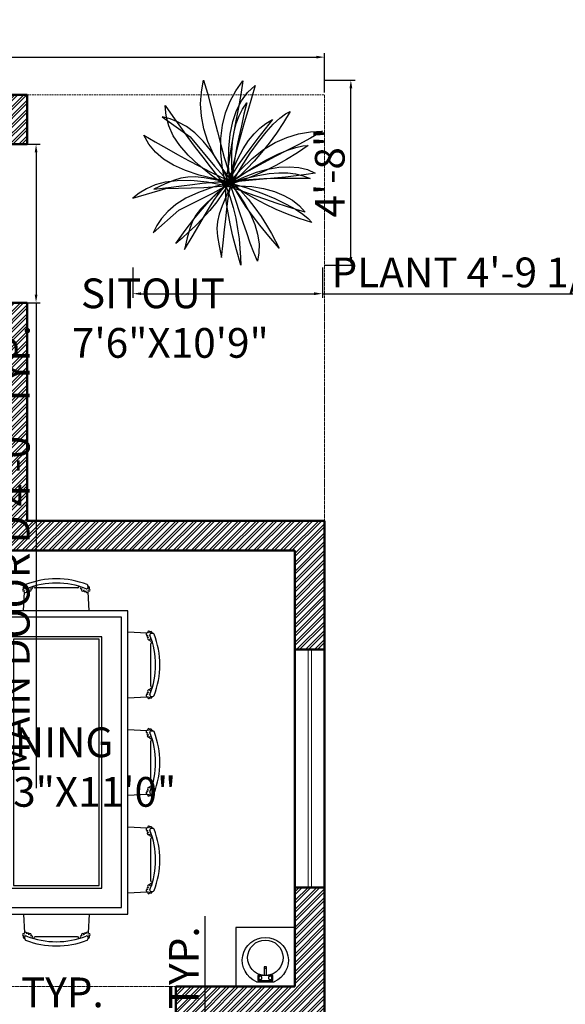
# Model space of a CAD drawing. Units: inches. Extents: x 3590 to 5167, y 65 to 1917.
# Tile 22 of 100: x 4213 to 4378, y 1531 to 1829. Entities that reach past the tile are written whole.
import ezdxf

# ---------------------------------------------------------------- set-up
doc = ezdxf.new("R2010")
doc.units = ezdxf.units.IN
doc.linetypes.add('DASHED', pattern=[0.75, 0.5, -0.25])
for name, color, linetype, lineweight in [('A-ANNO-DIMS', 2, 'Continuous', 18), ('A-AREA-IDEN', 7, 'Continuous', 18), ('A-FLOR-FIXT', 8, 'Continuous', 18), ('A-FURN', 21, 'Continuous', 18), ('A-GLAZ', 4, 'Continuous', 18), ('A-WALL', 7, 'Continuous', 50), ('A-WALL-PATT', 251, 'Continuous', 13), ('L-PLNT', 94, 'Continuous', 18), ('S-BEAM-OVHD', 7, 'DASHED', 18)]:
    doc.layers.add(name, color=color, linetype=linetype, lineweight=lineweight)
for name, color, linetype in [('DIENHOA', 3, 'Continuous'), ('FUR', 42, 'Continuous'), ('HA', 9, 'Continuous'), ('SANTEH', 7, 'Continuous'), ('wood', 26, 'Continuous')]:
    doc.layers.add(name, color=color, linetype=linetype)
doc.styles.get("Standard").update_dxf_attribs({"font": 'arial.ttf'})
doc.dimstyles.new('ISO-25', dxfattribs={"dimtxt": 9, "dimasz": 2.5, "dimexe": 1.25, "dimexo": 0.625, "dimtad": 1, "dimdec": 1, "dimlunit": 3, "dimtxsty": 'Standard', "dimcen": 2.5, "dimadec": 0, "dimazin": 0, "dimtfac": 1, "dimtdec": 1, "dimtmove": 0, "dimatfit": 3, "dimfxl": 1, "dimarcsym": 0})

# ---------------------------------------------------------------- blocks, each defined once
blk = doc.blocks.new('*D5')
at = {"layer": 'A-ANNO-DIMS', "color": 0, "lineweight": -2, "transparency": 16777216}
for p, q in [((3645.51, 1806.62), (3645.51, 1818.61)), ((4305.51, 1806.62), (4305.51, 1818.61)), ((3648.01, 1817.36), (4303.01, 1817.36))]:
    blk.add_line(p, q, dxfattribs=at)
at = {"layer": 'A-ANNO-DIMS', "color": 0, "transparency": 16777216}
for points in [[(3648.01, 1817.78), (3648.01, 1816.95), (3645.51, 1817.36)], [(4303.01, 1817.78), (4303.01, 1816.95), (4305.51, 1817.36)]]:
    blk.add_solid(points, dxfattribs=at)
at = {"layer": 'Defpoints', "color": 0, "transparency": 16777216}
for p in [(4305.51, 1817.36), (3645.51, 1806), (4305.51, 1806)]:
    blk.add_point(p, dxfattribs=at)
at = {"layer": 'A-ANNO-DIMS', "color": 0, "transparency": 16777216, "insert": (3975.51, 1822.57), "char_height": 9, "attachment_point": 5}
blk.add_mtext("55'", dxfattribs=at)
blk = doc.blocks.new('Cay03_mb')
at = {"layer": 'DIENHOA'}
for p, q in [((79.5, 503.7), (118.6, 555.3)), ((118.6, 555.3), (166.2, 599.1)), ((166.2, 599.1), (142.2, 519.4)), ((48.6, 443.6), (79.5, 503.7)), ((142.2, 519.4), (119, 441.7)), ((25.5, 374.3), (48.6, 443.6)), ((119, 441.7), (96.7, 365.6)), ((-365.2, 390.3), (-414.4, 402.8)), ((-414.4, 402.8), (-240.2, 277.8)), ((-314.9, 371.3), (-365.2, 390.3)), ((-263.5, 343.5), (-314.9, 371.3)), ((9.9, 295.3), (25.5, 374.3)), ((-211.2, 304.6), (-263.5, 343.5)), ((96.7, 365.6), (75.6, 290.6)), ((436.8, 297.2), (511, 309.6)), ((511, 309.6), (585.9, 313.5)), ((585.9, 313.5), (511.8, 271.4)), ((-240.2, 277.8), (-88.4, 94.9)), ((-158, 252.3), (-211.2, 304.6)), ((-104.2, 184.4), (-158, 252.3)), ((1.6, 205.7), (9.9, 295.3)), ((75.6, 290.6), (55.7, 216.3)), ((290.6, 243.2), (363.4, 275.4)), ((363.4, 275.4), (436.8, 297.2)), ((511.8, 271.4), (437.6, 231.5)), ((0.2, 104.9), (1.6, 205.7)), ((55.7, 216.3), (37.3, 142.1)), ((147, 144.1), (218.5, 199.8)), ((218.5, 199.8), (290.6, 243.2)), ((363.7, 192.9), (290.2, 154.9)), ((437.6, 231.5), (363.7, 192.9)), ((-49.6, 98.5), (-104.2, 184.4)), ((37.3, 142.1), (20.5, 67.6)), ((75.9, 75.2), (147, 144.1)), ((290.2, 154.9), (217.4, 116.6)), ((-88.4, 94.9), (5.4, -7.8)), ((5.4, -7.8), (-49.6, 98.5)), ((5.4, -7.8), (0.2, 104.9)), ((5.4, -7.8), (75.9, 75.2)), ((20.5, 67.6), (5.4, -7.8)), ((145.5, 77.3), (74.7, 36.1)), ((217.4, 116.6), (145.5, 77.3)), ((-345, 5.4), (-399.6, -17.1)), ((-298.6, 20.1), (-345, 5.4)), ((-254.7, 27.4), (-298.6, 20.1)), ((-208, 27.8), (-254.7, 27.4)), ((-152.7, 21.7), (-208, 27.8)), ((-83.4, 9.7), (-152.7, 21.7)), ((5.4, -7.8), (-83.4, 9.7)), ((74.7, 36.1), (5.4, -7.8)), ((5.4, -7.8), (100.3, 18.4)), ((46.3, 0.9), (5.4, -7.8)), ((96.7, 7.5), (46.3, 0.9)), ((155, 12.2), (96.7, 7.5)), ((100.3, 18.4), (182.2, 37.2)), ((219.6, 15.4), (155, 12.2)), ((182.2, 37.2), (253, 48.9)), ((289, 17.4), (219.6, 15.4)), ((253, 48.9), (314.6, 54.1)), ((361.6, 18.5), (289, 17.4)), ((314.6, 54.1), (369.2, 53.3)), ((435.8, 18.9), (361.6, 18.5)), ((369.2, 53.3), (418.6, 46.8)), ((418.6, 46.8), (464.9, 35.2)), ((510, 19), (435.8, 18.9)), ((464.9, 35.2), (510, 19)), ((-399.6, -17.1), (-468, -47.9)), ((-468, -47.9), (-375.6, -37.8)), ((-375.6, -37.8), (-295.3, -27.9)), ((-295.3, -27.9), (-225.8, -18.9)), ((-225.8, -18.9), (-165.8, -11.3)), ((-165.8, -11.3), (-114, -5.7)), ((-114, -5.7), (-69, -2.9)), ((-79.8, -79.6), (-45.1, -46.3)), ((-69, -2.9), (-29.6, -3.4)), ((-45.1, -46.3), (-16.5, -22.4)), ((5.4, -7.8), (-33.2, -69.5)), ((-29.6, -3.4), (5.4, -7.8)), ((-16.5, -22.4), (5.4, -7.8)), ((5.4, -7.8), (56.8, -73.3)), ((25.9, -64.4), (5.4, -7.8)), ((5.4, -7.8), (112.8, -40.3)), ((53.5, -41.6), (5.4, -7.8)), ((107, -75.7), (53.5, -41.6)), ((112.8, -40.3), (207.5, -73.8)), ((-165.9, -174.1), (-120.2, -122.1)), ((-120.2, -122.1), (-79.8, -79.6)), ((-33.2, -69.5), (-74.6, -127.3)), ((47, -125.9), (25.9, -64.4)), ((56.8, -73.3), (100.4, -139.1)), ((165.5, -109.6), (107, -75.7)), ((228.7, -142.8), (165.5, -109.6)), ((207.5, -73.8), (289.5, -107.6)), ((289.5, -107.6), (359.3, -141.1)), ((-216.3, -235.6), (-165.9, -174.1)), ((-117.8, -181.1), (-162.1, -230.9)), ((-74.6, -127.3), (-117.8, -181.1)), ((68.7, -190.6), (47, -125.9)), ((100.4, -139.1), (135.9, -204.3)), ((296, -174.7), (228.7, -142.8)), ((367.1, -204.8), (296, -174.7)), ((359.3, -141.1), (416.9, -173.5)), ((416.9, -173.5), (462.6, -204.2)), ((-271, -306.6), (-216.3, -235.6)), ((-162.1, -230.9), (-206.3, -276.5)), ((90.8, -256.6), (68.7, -190.6)), ((135.9, -204.3), (162.8, -268.3)), ((441.6, -232.7), (367.1, -204.8)), ((518.9, -257.7), (441.6, -232.7)), ((462.6, -204.2), (496.5, -232.5)), ((496.5, -232.5), (518.9, -257.7)), ((-329.5, -387.1), (-271, -306.6)), ((-206.3, -276.5), (-249.6, -317.8)), ((113.1, -322.2), (90.8, -256.6)), ((162.8, -268.3), (181, -330.4)), ((-291, -354.7), (-329.5, -387.1)), ((-249.6, -317.8), (-291, -354.7)), ((135.4, -385.6), (113.1, -322.2)), ((181, -330.4), (190, -390)), ((157.6, -445), (135.4, -385.6)), ((190, -390), (189.6, -446.3)), ((179.5, -498.7), (157.6, -445)), ((189.6, -446.3), (179.5, -498.7))]:
    blk.add_line(p, q, dxfattribs=at)
for points in [[(23.7, -5.4), (-41, 82.2), (-91.8, 167.1), (-129.7, 249.5), (-155.6, 329.6), (-170.2, 407.8), (-174.7, 484.2), (-169.8, 559.3), (-156.5, 633.1)], [(-156.5, 633.1), (-132.5, 551.3), (-110.5, 470), (-89.8, 389.2), (-69.6, 309), (-49, 229.4), (-27.1, 150.4), (-3.2, 72.1), (23.7, -5.4)], [(-16.4, -26.7), (-38.3, 80), (-48.9, 178.3), (-48.7, 269), (-38.5, 352.6), (-19.1, 429.7), (9, 501), (44.9, 567.1), (87.9, 628.5)], [(87.9, 628.5), (75.5, 544.2), (61.3, 461.2), (46.1, 379.1), (30.8, 297.8), (16.1, 216.9), (2.9, 136), (-8.3, 54.9), (-16.4, -26.7)], [(-395.6, 473.7), (-347.5, 405.6), (-300.6, 339.5), (-254.3, 275.1), (-208.3, 212.3), (-161.9, 150.9), (-114.8, 90.7), (-66.5, 31.6), (-16.4, -26.7)], [(-16.4, -26.7), (-108.3, 38.6), (-186.9, 101.7), (-252.4, 163.5), (-305.1, 224.4), (-345.4, 285.2), (-373.7, 346.6), (-390.4, 409.2), (-395.6, 473.7)], [(23.7, -5.4), (19.8, 93), (20.3, 177), (25, 248.5), (34, 309.8), (47.3, 362.7), (64.9, 409.3), (86.8, 451.7), (112.9, 491.9)], [(112.9, 491.9), (96, 419.7), (79.5, 347.4), (63.9, 276.5), (50, 208.4), (38.4, 144.8), (29.7, 86.9), (24.6, 36.3), (23.7, -5.4)], [(384.3, 437.5), (342.2, 367.8), (298.1, 301.7), (252.6, 239.4), (206.1, 181.1), (159.4, 127.2), (113, 78), (67.6, 33.6), (23.7, -5.4)], [(23.7, -5.4), (79.9, 91.7), (134.1, 176.2), (185.8, 248.4), (234.3, 308.7), (279, 357.3), (319.3, 394.8), (354.6, 421.4), (384.3, 437.5)], [(273.2, 387.3), (227.6, 328.8), (182.3, 270.1), (138.4, 212.3), (97.2, 156.4), (60, 103.4), (27.8, 54.6), (1.9, 10.8), (-16.4, -26.7)], [(-16.4, -26.7), (21.4, 64.2), (57, 140.3), (91.4, 203.3), (125.2, 255.1), (159.5, 297.5), (195, 332.5), (232.7, 361.8), (273.2, 387.3)], [(-530.5, 289.7), (-458.3, 248.1), (-387.9, 207.8), (-318.9, 168.7), (-250.8, 131.1), (-182.9, 94.8), (-114.9, 59.9), (-46.2, 26.5), (23.7, -5.4)], [(23.7, -5.4), (-87.2, 15.2), (-185, 39.6), (-270.3, 68.2), (-343.7, 101.4), (-405.9, 139.7), (-457.3, 183.5), (-498.7, 233.4), (-530.5, 289.7)], [(496.7, 224), (429.4, 178.4), (361.6, 136.9), (294.1, 99.5), (227.5, 66.1), (162.4, 36.7), (99.7, 11.5), (39.8, -9.7), (-16.4, -26.7)], [(-16.4, -26.7), (75.4, 37.9), (160.1, 91.8), (237.3, 135.7), (306.6, 170), (367.6, 195.4), (419.9, 212.5), (463.1, 221.9), (496.7, 224)], [(23.7, -5.4), (99.3, 29.7), (173.2, 57.1), (244.8, 76.7), (313.3, 88.3), (377.9, 91.8), (437.9, 87), (492.7, 73.8), (541.4, 52)], [(-16.4, -26.7), (-134, -4.7), (-235.3, 5.3), (-322, 4.7), (-395.9, -5), (-458.7, -22.3), (-512.3, -45.7), (-558.2, -73.6), (-598.4, -104.7)], [(541.4, 52), (484.1, 42.9), (421.2, 34.8), (354.4, 27.6), (285.4, 20.9), (216.1, 14.5), (148.2, 8.1), (83.5, 1.6), (23.7, -5.4)], [(-598.4, -104.7), (-392.7, -44.4), (-155, -37.4), (-16.4, -26.7)], [(-471.9, -320.3), (-310.5, -179.3), (-97.7, -73.3), (23.7, -5.4)], [(23.7, -5.4), (-92.3, -34.8), (-188.4, -68.2), (-266.9, -105.1), (-329.9, -144.9), (-379.7, -187), (-418.5, -230.7), (-448.5, -275.3), (-471.9, -320.3)], [(-276.2, -424.4), (-227.3, -345.4), (-185.7, -276.1), (-150, -215.7), (-119.1, -163.8), (-91.5, -119.5), (-66, -82.3), (-41.4, -51.6), (-16.4, -26.7)], [(-16.4, -26.7), (-84.9, -86), (-137, -133.1), (-175.8, -173), (-204.3, -210), (-225.5, -249.1), (-242.5, -294.7), (-258.4, -351.6), (-276.2, -424.4)], [(23.7, -5.4), (-13.6, -87.9), (-41.1, -152.6), (-59.6, -205), (-69.9, -250.7), (-72.8, -295), (-69.2, -343.6), (-59.7, -401.9), (-45.3, -475.5)], [(-45.3, -475.5), (-34.1, -383.2), (-25.4, -302.8), (-18.3, -233.1), (-12, -172.9), (-5.6, -121.2), (2, -76.8), (11.4, -38.5), (23.7, -5.4)], [(76.2, -524.2), (48.8, -428.5), (26.6, -341.7), (9.2, -264.1), (-3.6, -196.1), (-12.3, -138), (-17.1, -90.2), (-18.3, -53), (-16.4, -26.7)], [(-16.4, -26.7), (66.9, -26.6), (145.6, -32.7), (218.8, -44.9), (285.8, -63.1), (345.9, -87.1), (398.4, -116.6), (442.6, -151.6), (477.6, -191.8)], [(477.6, -191.8), (421.8, -176), (361.3, -156.9), (297.6, -135.5), (232.2, -112.6), (166.6, -89.4), (102.3, -66.6), (40.8, -45.4), (-16.4, -26.7)], [(-16.4, -26.7), (8.5, -95.1), (28.5, -163.3), (44.3, -230.6), (56.3, -296.1), (65, -359), (70.9, -418.5), (74.5, -473.9), (76.2, -524.2)], [(316.5, -418.1), (251.4, -342.8), (194.8, -273.3), (146.5, -210.2), (106.3, -153.8), (74.1, -104.7), (49.7, -63.4), (32.9, -30.1), (23.7, -5.4)], [(23.7, -5.4), (74.9, -57.1), (121.8, -110.6), (164.3, -165), (202.7, -219.4), (237, -272.9), (267.3, -324.5), (293.7, -373.2), (316.5, -418.1)]]:
    blk.add_lwpolyline(points, dxfattribs=at)
blk = doc.blocks.new('A$C39F63D19')
at = {"layer": 'FUR'}
for p, q in [((1.415, 2.4468), (1.4061, 2.4547)), ((1.5486, 2.3264), (1.4408, 2.4235)), ((1.3599, 2.3864), (1.1308, 2.1573)), ((1.3599, 2.4017), (1.3588, 2.4028)), ((2.0077, 2.3522), (2.0166, 2.3602)), ((1.8741, 2.2319), (1.9819, 2.329)), ((2.0628, 2.3072), (2.0639, 2.3083)), ((2.0628, 2.2919), (2.2919, 2.0628)), ((1.1155, 2.1573), (1.1144, 2.1585)), ((1.1155, 2.1573), (1.1144, 2.1585)), ((1.0705, 2.1023), (1.0625, 2.1111)), ((1.1908, 1.9686), (1.0937, 2.0765)), ((2.3072, 2.0628), (2.3083, 2.0639)), ((2.3072, 2.0628), (2.3083, 2.0639)), ((2.2319, 1.8741), (2.329, 1.9819)), ((2.3522, 2.0077), (2.3602, 2.0166)), ((0.8846, 1.9165), (0.8758, 1.9244)), ((1.0183, 1.7961), (0.9104, 1.8932)), ((0.8296, 1.8561), (0.6005, 1.627)), ((0.8296, 1.8714), (0.8285, 1.8725)), ((0.5852, 1.627), (0.5841, 1.6281)), ((0.5852, 1.627), (0.5841, 1.6281)), ((0.5401, 1.572), (0.5322, 1.5808)), ((0.6605, 1.4383), (0.5634, 1.5462)), ((2.3264, 1.5486), (2.4235, 1.4408)), ((0.3543, 1.3861), (0.3455, 1.3941)), ((0.488, 1.2658), (0.3801, 1.3629)), ((2.4468, 1.415), (2.4547, 1.4061)), ((0.2993, 1.3258), (0.0701, 1.0967)), ((0.2993, 1.3411), (0.2981, 1.3422)), ((2.3864, 1.3599), (2.1573, 1.1308)), ((2.4017, 1.3599), (2.4028, 1.3588)), ((1.9686, 1.1908), (2.0765, 1.0937)), ((0.0549, 1.0967), (0.0538, 1.0978)), ((0.0549, 1.0967), (0.0538, 1.0978)), ((2.1023, 1.0705), (2.1111, 1.0625)), ((2.1573, 1.1155), (2.1585, 1.1144)), ((2.1573, 1.1155), (2.1585, 1.1144)), ((0.0098, 1.0416), (0.0019, 1.0505)), ((0.1302, 0.908), (0.033, 1.0158)), ((1.7961, 1.0183), (1.8932, 0.9104)), ((1.9165, 0.8846), (1.9244, 0.8758)), ((1.8561, 0.8296), (1.627, 0.6005)), ((1.8714, 0.8296), (1.8725, 0.8285)), ((1.4383, 0.6605), (1.5462, 0.5634)), ((0.2247, 0.5825), (0.1276, 0.4747)), ((1.572, 0.5401), (1.5808, 0.5322)), ((1.627, 0.5852), (1.6281, 0.5841)), ((1.627, 0.5852), (1.6281, 0.5841)), ((1.2658, 0.488), (1.3629, 0.3801)), ((0.1044, 0.4489), (0.0964, 0.44)), ((0.1494, 0.3938), (0.1483, 0.3927)), ((0.1647, 0.3938), (0.3938, 0.1647)), ((1.3861, 0.3543), (1.3941, 0.3455)), ((1.3258, 0.2993), (1.0967, 0.0701)), ((1.3411, 0.2993), (1.3422, 0.2981)), ((0.5825, 0.2247), (0.4747, 0.1276)), ((0.3938, 0.1494), (0.3927, 0.1483)), ((0.3938, 0.1494), (0.3927, 0.1483)), ((0.4489, 0.1044), (0.44, 0.0964)), ((0.908, 0.1302), (1.0158, 0.033)), ((1.0416, 0.0098), (1.0505, 0.0019)), ((1.0967, 0.0549), (1.0978, 0.0538)), ((1.0967, 0.0549), (1.0978, 0.0538))]:
    blk.add_line(p, q, dxfattribs=at)
for points in [[(1.6641, 2.4419), (0.0147, 0.7925), (0.7925, 0.0147), (2.4419, 1.6641)], [(1.6641, 2.3712), (0.0854, 0.7925), (0.7925, 0.0854), (2.3712, 1.6641)], [(1.6641, 2.159), (0.2976, 0.7925), (0.7925, 0.2976), (2.159, 1.6641)]]:
    blk.add_lwpolyline(points, close=True, dxfattribs=at)
for centre, radius, start, end in [((1.6574, 1.8598), 0.6521, 113.77302, 156.22698), ((1.6574, 1.8598), 0.6197, 113.33062, 156.66938), ((1.3989, 2.4467), 0.0108, 48, 113.77302), ((1.4185, 2.4458), 0.0101, 329.62103, 147.42526), ((1.4077, 2.4388), 0.0108, 293.33062, 48), ((1.4308, 2.4208), 0.0103, 213.3009, 71.36297), ((1.4349, 2.4385), 0.00795, 264.76881, 163.65384), ((1.3523, 2.3941), 0.0108, 315, 45), ((1.3814, 2.4068), 0.0085, 151.04971, 5.85435), ((1.3995, 2.4044), 0.0102, 161.25601, 35.99509), ((1.4156, 2.411), 0.00785, 184.4301, 31.81325), ((1.9878, 2.3439), 0.00795, 16.34616, 275.23119), ((2.0042, 2.3512), 0.0101, 32.57474, 210.37897), ((2.015, 2.3442), 0.0108, 132, 246.66938), ((2.0238, 2.3521), 0.0108, 66.22698, 132), ((1.7653, 1.7653), 0.6521, 23.77302, 66.22698), ((1.9919, 2.3262), 0.0103, 108.63703, 326.6991), ((2.0071, 2.3164), 0.00785, 148.18675, 355.5699), ((1.7653, 1.7653), 0.6197, 23.33062, 66.66938), ((2.0232, 2.3098), 0.0102, 144.00491, 18.74399), ((2.0413, 2.3122), 0.0085, 174.14565, 28.95029), ((2.0704, 2.2995), 0.0108, 135, 225), ((1.0705, 2.1184), 0.0108, 156.22698, 222), ((1.1105, 2.1359), 0.0085, 264.14565, 118.95029), ((1.1232, 2.165), 0.0108, 225, 315), ((1.0715, 2.0987), 0.0101, 122.57474, 300.37897), ((1.0785, 2.1095), 0.0108, 222, 336.66938), ((1.0788, 2.0824), 0.00795, 106.34616, 5.23119), ((1.0965, 2.0864), 0.0103, 198.63703, 56.6991), ((1.1063, 2.1017), 0.00785, 238.18675, 85.5699), ((2.2995, 2.0704), 0.0108, 225, 315), ((2.3122, 2.0413), 0.0085, 61.04971, 275.85435), ((2.3098, 2.0232), 0.0102, 71.25601, 305.99509), ((2.3164, 2.0071), 0.00785, 94.4301, 301.81325), ((2.3262, 1.9919), 0.0103, 123.3009, 341.36297), ((2.3442, 2.015), 0.0108, 203.33062, 318), ((2.3439, 1.9878), 0.00795, 174.76881, 73.65384), ((2.3512, 2.0042), 0.0101, 239.62103, 57.42526), ((2.3521, 2.0238), 0.0108, 318, 23.77302), ((1.1271, 1.3295), 0.6521, 113.77302, 156.22698), ((1.1271, 1.3295), 0.6197, 113.33062, 156.66938), ((0.8686, 1.9164), 0.0108, 48, 113.77302), ((0.8882, 1.9155), 0.0101, 329.62103, 147.42526), ((0.8774, 1.9084), 0.0108, 293.33062, 48), ((0.9005, 1.8904), 0.0103, 213.3009, 71.36297), ((0.9045, 1.9081), 0.00795, 264.76881, 163.65384), ((0.8219, 1.8638), 0.0108, 315, 45), ((0.8511, 1.8765), 0.0085, 151.04971, 5.85435), ((0.8692, 1.8741), 0.0102, 161.25601, 35.99509), ((0.8852, 1.8806), 0.00785, 184.4301, 31.81325), ((0.5402, 1.588), 0.0108, 156.22698, 222), ((0.5801, 1.6055), 0.0085, 264.14565, 118.95029), ((0.5825, 1.5874), 0.0102, 234.00491, 108.74399), ((0.5928, 1.6347), 0.0108, 225, 315), ((0.5411, 1.5684), 0.0101, 122.57474, 300.37897), ((0.5482, 1.5792), 0.0108, 222, 336.66938), ((0.5485, 1.5521), 0.00795, 106.34616, 5.23119), ((0.5662, 1.5561), 0.0103, 198.63703, 56.6991), ((0.576, 1.5714), 0.00785, 238.18675, 85.5699), ((2.4208, 1.4308), 0.0103, 18.63703, 236.6991), ((2.4385, 1.4349), 0.00795, 286.34616, 185.23119), ((0.5968, 0.7992), 0.6521, 113.77302, 156.22698), ((0.5968, 0.7992), 0.6197, 113.33062, 156.66938), ((0.3382, 1.3861), 0.0108, 48, 113.77302), ((0.3579, 1.3851), 0.0101, 329.62103, 147.42526), ((0.3471, 1.3781), 0.0108, 293.33062, 48), ((0.3702, 1.3601), 0.0103, 213.3009, 71.36297), ((0.3742, 1.3778), 0.00795, 264.76881, 163.65384), ((1.8598, 1.6574), 0.6197, 293.33062, 336.66938), ((1.8598, 1.6574), 0.6521, 293.77302, 336.22698), ((2.3941, 1.3523), 0.0108, 45, 135), ((2.4044, 1.3995), 0.0102, 54.00491, 288.74399), ((2.4068, 1.3814), 0.0085, 84.14565, 298.95029), ((2.411, 1.4156), 0.00785, 58.18675, 265.5699), ((2.4388, 1.4077), 0.0108, 42, 156.66938), ((2.4458, 1.4185), 0.0101, 302.57474, 120.37897), ((2.4467, 1.3989), 0.0108, 336.22698, 42), ((0.2916, 1.3334), 0.0108, 315, 45), ((0.3207, 1.3461), 0.0085, 151.04971, 5.85435), ((0.3388, 1.3437), 0.0102, 161.25601, 35.99509), ((0.3549, 1.3503), 0.00785, 184.4301, 31.81325), ((0.0099, 1.0577), 0.0108, 156.22698, 222), ((0.0498, 1.0752), 0.0085, 264.14565, 118.95029), ((0.0522, 1.0571), 0.0102, 234.00491, 108.74399), ((0.0625, 1.1043), 0.0108, 225, 315), ((2.0824, 1.0788), 0.00795, 84.76881, 343.65384), ((2.0864, 1.0965), 0.0103, 33.3009, 251.36297), ((2.0987, 1.0715), 0.0101, 149.62103, 327.42526), ((2.1017, 1.1063), 0.00785, 4.4301, 211.81325), ((2.1095, 1.0785), 0.0108, 113.33062, 228), ((2.1178, 1.1129), 0.0102, 341.25601, 215.99509), ((2.1184, 1.0705), 0.0108, 228, 293.77302), ((2.1359, 1.1105), 0.0085, 331.04971, 185.85435), ((2.165, 1.1232), 0.0108, 135, 225), ((0.0108, 1.0381), 0.0101, 122.57474, 300.37897), ((0.0178, 1.0489), 0.0108, 222, 336.66938), ((0.0181, 1.0217), 0.00795, 106.34616, 5.23119), ((0.0358, 1.0258), 0.0103, 198.63703, 56.6991), ((0.0456, 1.041), 0.00785, 238.18675, 85.5699), ((1.8904, 0.9005), 0.0103, 18.63703, 236.6991), ((1.9081, 0.9045), 0.00795, 286.34616, 185.23119), ((1.3295, 1.1271), 0.6197, 293.33062, 336.66938), ((1.3295, 1.1271), 0.6521, 293.77302, 336.22698), ((1.8741, 0.8692), 0.0102, 54.00491, 288.74399), ((1.8765, 0.8511), 0.0085, 84.14565, 298.95029), ((1.8806, 0.8852), 0.00785, 58.18675, 265.5699), ((1.9084, 0.8774), 0.0108, 42, 156.66938), ((1.9155, 0.8882), 0.0101, 302.57474, 120.37897), ((1.9164, 0.8686), 0.0108, 336.22698, 42), ((1.8638, 0.8219), 0.0108, 45, 135), ((1.5521, 0.5485), 0.00795, 84.76881, 343.65384), ((1.5561, 0.5662), 0.0103, 33.3009, 251.36297), ((1.5684, 0.5411), 0.0101, 149.62103, 327.42526), ((1.5714, 0.576), 0.00785, 4.4301, 211.81325), ((1.5792, 0.5482), 0.0108, 113.33062, 228), ((1.5874, 0.5825), 0.0102, 341.25601, 215.99509), ((1.588, 0.5402), 0.0108, 228, 293.77302), ((1.6055, 0.5801), 0.0085, 331.04971, 185.85435), ((1.6347, 0.5928), 0.0108, 135, 225), ((0.1054, 0.4524), 0.0101, 59.62103, 237.42526), ((0.1127, 0.4688), 0.00795, 354.76881, 253.65384), ((0.1304, 0.4647), 0.0103, 303.3009, 161.36297), ((0.1402, 0.4495), 0.00785, 274.4301, 121.81325), ((0.1044, 0.4328), 0.0108, 138, 203.77302), ((0.6913, 0.6913), 0.6521, 203.77302, 246.22698), ((0.1124, 0.4416), 0.0108, 23.33062, 138), ((0.6913, 0.6913), 0.6197, 203.33062, 246.66938), ((0.1444, 0.4153), 0.0085, 241.04971, 95.85435), ((0.1468, 0.4334), 0.0102, 251.25601, 125.99509), ((0.1571, 0.3862), 0.0108, 45, 135), ((1.3601, 0.3702), 0.0103, 18.63703, 236.6991), ((1.3778, 0.3742), 0.00795, 286.34616, 185.23119), ((0.7992, 0.5968), 0.6197, 293.33062, 336.66938), ((0.7992, 0.5968), 0.6521, 293.77302, 336.22698), ((1.3437, 0.3388), 0.0102, 54.00491, 288.74399), ((1.3461, 0.3207), 0.0085, 84.14565, 298.95029), ((1.3503, 0.3549), 0.00785, 58.18675, 265.5699), ((1.3781, 0.3471), 0.0108, 42, 156.66938), ((1.3851, 0.3579), 0.0101, 302.57474, 120.37897), ((1.3861, 0.3382), 0.0108, 336.22698, 42), ((1.3334, 0.2916), 0.0108, 45, 135), ((0.3862, 0.1571), 0.0108, 315, 45), ((0.4153, 0.1444), 0.0085, 354.14565, 208.95029), ((0.4334, 0.1468), 0.0102, 324.00491, 198.74399), ((0.4328, 0.1044), 0.0108, 246.22698, 312), ((0.4495, 0.1402), 0.00785, 328.18675, 175.5699), ((0.4524, 0.1054), 0.0101, 212.57474, 30.37897), ((0.4416, 0.1124), 0.0108, 312, 66.66938), ((0.4647, 0.1304), 0.0103, 288.63703, 146.6991), ((0.4688, 0.1127), 0.00795, 196.34616, 95.23119), ((1.0217, 0.0181), 0.00795, 84.76881, 343.65384), ((1.0258, 0.0358), 0.0103, 33.3009, 251.36297), ((1.0381, 0.0108), 0.0101, 149.62103, 327.42526), ((1.041, 0.0456), 0.00785, 4.4301, 211.81325), ((1.0489, 0.0178), 0.0108, 113.33062, 228), ((1.0571, 0.0522), 0.0102, 341.25601, 215.99509), ((1.0577, 0.0099), 0.0108, 228, 293.77302), ((1.0752, 0.0498), 0.0085, 331.04971, 185.85435), ((1.1043, 0.0625), 0.0108, 135, 225)]:
    blk.add_arc(centre, radius, start, end, dxfattribs=at)
at = {"layer": 'HA'}
blk.add_lwpolyline([(1.6641, 2.1308), (0.3258, 0.7925), (0.7925, 0.3258), (2.1308, 1.6641)], close=True, dxfattribs=at)
at = {"layer": 'wood'}
for points in [[(1.3825, 2.4152, 0.308332), (1.374, 2.4109, -0.00386)], [(1.4096, 2.4059, -0.15729), (1.4077, 2.4104, -0.120016)], [(1.1113, 2.1077, 1.044756), (1.1135, 2.1279, -0.117685), (1.1096, 2.1274, -1.643727), (1.1069, 2.1095, -0.15729)], [(2.3158, 2.015, -0.120016), (2.3113, 2.0131, -0.15729)], [(0.8522, 1.8849, 0.308332), (0.8436, 1.8806, -0.00386)], [(0.8792, 1.8756, -0.15729), (0.8774, 1.88, -0.120016)], [(0.581, 1.5774, 1.044756), (0.5832, 1.5976, -0.117685), (0.5793, 1.5971, -1.643727), (0.5766, 1.5792, -0.15729)], [(2.4104, 1.4077, -0.15729), (2.4059, 1.4096, 1.044756), (2.4037, 1.3893, -0.117685), (2.4077, 1.3899, -1.643727)], [(0.3489, 1.3453, -0.15729), (0.3471, 1.3497, -0.120016)], [(2.1095, 1.1069, -0.120016), (2.1077, 1.1113, -0.15729)], [(2.1347, 1.102, 0.308332), (2.1433, 1.1064, -0.00386)], [(1.88, 0.8774, -0.15729), (1.8756, 0.8792, 1.044756), (1.8734, 0.859, -0.117685), (1.8773, 0.8595, -1.643727)], [(1.5792, 0.5766, -0.120016), (1.5774, 0.581, -0.15729)], [(1.6044, 0.5717, 0.308332), (1.613, 0.576, -0.00386)], [(0.1453, 0.4435, -0.15729), (0.1408, 0.4416, -0.120016)], [(1.3497, 0.3471, -0.15729), (1.3453, 0.3489, 1.044756), (1.3431, 0.3287, -0.117685), (1.347, 0.3292, -1.643727)], [(1.0489, 0.0462, -0.120016), (1.047, 0.0507, -0.15729)], [(1.0741, 0.0414, 0.308332), (1.0826, 0.0457, -0.00386)]]:
    blk.add_lwpolyline(points, format="xyb", close=True, dxfattribs=at)
blk = doc.blocks.new('r11')
at = {"layer": 'SANTEH', "ltscale": 5}
for p, q in [((0, 0), (600, 0)), ((0, -600), (0, 0)), ((600, 0), (600, -600)), ((210, -50), (390, -50)), ((210, -50), (210, -50)), ((224, -63), (376, -63)), ((224, -113), (224, -63)), ((233, -79), (249, -69)), ((233, -98), (233, -79)), ((249, -107), (233, -98)), ((249, -69), (266, -79)), ((266, -98), (249, -107)), ((266, -79), (266, -98)), ((334, -79), (351, -69)), ((334, -98), (334, -79)), ((351, -107), (334, -98)), ((351, -69), (367, -79)), ((367, -98), (351, -107)), ((367, -79), (367, -98)), ((376, -63), (376, -113)), ((376, -113), (224, -113)), ((288, -202), (288, -113)), ((312, -184), (288, -184)), ((312, -113), (312, -202)), ((312, -202), (288, -202)), ((600, -600), (0, -600))]:
    blk.add_line(p, q, dxfattribs=at)
for centre, radius, start, end in [((300, -266), 234, 112.5, 67.5), ((300, -293), 180, 93.8183, 86.1817)]:
    blk.add_arc(centre, radius, start, end, dxfattribs=at)
blk = doc.blocks.new('*D294')
at = {"layer": 'A-ANNO-DIMS', "color": 0, "lineweight": -2, "transparency": 16777216}
for p, q in [((3946.19, 1546.03), (3946.19, 1526.56)), ((4071.76, 1546.03), (4071.76, 1526.56)), ((3948.69, 1527.81), (4069.26, 1527.81)), ((4071.76, 1527.81), (4243.57, 1527.81))]:
    blk.add_line(p, q, dxfattribs=at)
at = {"layer": 'A-ANNO-DIMS', "color": 0, "transparency": 16777216}
for points in [[(3948.69, 1528.23), (3948.69, 1527.4), (3946.19, 1527.81)], [(4069.26, 1528.23), (4069.26, 1527.4), (4071.76, 1527.81)]]:
    blk.add_solid(points, dxfattribs=at)
at = {"layer": 'Defpoints', "color": 0, "transparency": 16777216}
for p in [(3946.19, 1546.65), (4071.76, 1546.65), (4071.76, 1527.81)]:
    blk.add_point(p, dxfattribs=at)
at = {"layer": 'A-ANNO-DIMS', "color": 0, "transparency": 16777216, "insert": (4158.91, 1533.1), "char_height": 9, "attachment_point": 5}
blk.add_mtext('3-SEAT SOFA 10\'-5 1/2" TYP.', dxfattribs=at)
blk = doc.blocks.new('*D308')
at = {"layer": 'A-ANNO-DIMS', "color": 0, "lineweight": -2, "transparency": 16777216}
for p, q in [((4269.39, 1429.97), (4269.39, 1557.29)), ((4272.58, 1429.97), (4268.14, 1429.97)), ((4269.39, 1407.01), (4269.39, 1427.47)), ((4272.58, 1404.51), (4268.14, 1404.51))]:
    blk.add_line(p, q, dxfattribs=at)
at = {"layer": 'A-ANNO-DIMS', "color": 0, "transparency": 16777216}
for points in [[(4268.97, 1427.47), (4269.8, 1427.47), (4269.39, 1429.97)], [(4268.97, 1407.01), (4269.8, 1407.01), (4269.39, 1404.51)]]:
    blk.add_solid(points, dxfattribs=at)
at = {"layer": 'Defpoints', "color": 0, "transparency": 16777216}
for p in [(4269.39, 1429.97), (4273.2, 1429.97), (4273.2, 1404.51)]:
    blk.add_point(p, dxfattribs=at)
at = {"layer": 'A-ANNO-DIMS', "color": 0, "transparency": 16777216, "insert": (4264.11, 1494.88), "char_height": 9, "attachment_point": 5, "rotation": 90}
blk.add_mtext('RANGE 2\'-1 1/2" TYP.', dxfattribs=at)
blk = doc.blocks.new('*D316')
at = {"layer": 'A-ANNO-DIMS', "color": 0, "lineweight": -2, "transparency": 16777216}
for p, q in [((4211.64, 1791), (4219.46, 1791)), ((4218.21, 1788.5), (4218.21, 1745.5)), ((4211.64, 1743), (4219.46, 1743)), ((4218.21, 1743), (4218.21, 1596.09))]:
    blk.add_line(p, q, dxfattribs=at)
at = {"layer": 'A-ANNO-DIMS', "color": 0, "transparency": 16777216}
for points in [[(4217.8, 1788.5), (4218.63, 1788.5), (4218.21, 1791)], [(4217.8, 1745.5), (4218.63, 1745.5), (4218.21, 1743)]]:
    blk.add_solid(points, dxfattribs=at)
at = {"layer": 'Defpoints', "color": 0, "transparency": 16777216}
for p in [(4211.01, 1791), (4211.01, 1743), (4218.21, 1743)]:
    blk.add_point(p, dxfattribs=at)
at = {"layer": 'A-ANNO-DIMS', "color": 0, "transparency": 16777216, "insert": (4212.93, 1668.29), "char_height": 9, "attachment_point": 5, "rotation": 90}
blk.add_mtext('MAIN DOOR D 4\'-0" TYP.', dxfattribs=at)
blk = doc.blocks.new('*D320')
at = {"layer": 'A-ANNO-DIMS', "color": 0, "lineweight": -2, "transparency": 16777216}
for p, q in [((4247.49, 1753.73), (4247.49, 1744.5)), ((4304.85, 1753.73), (4304.85, 1744.5)), ((4249.99, 1745.75), (4302.35, 1745.75)), ((4304.85, 1745.75), (4397.07, 1745.75))]:
    blk.add_line(p, q, dxfattribs=at)
at = {"layer": 'A-ANNO-DIMS', "color": 0, "transparency": 16777216}
for points in [[(4249.99, 1746.17), (4249.99, 1745.33), (4247.49, 1745.75)], [(4302.35, 1746.17), (4302.35, 1745.33), (4304.85, 1745.75)]]:
    blk.add_solid(points, dxfattribs=at)
at = {"layer": 'Defpoints', "color": 0, "transparency": 16777216}
for p in [(4247.49, 1754.35), (4304.85, 1754.35), (4304.85, 1745.75)]:
    blk.add_point(p, dxfattribs=at)
at = {"layer": 'A-ANNO-DIMS', "color": 0, "transparency": 16777216, "insert": (4352.21, 1751.03), "char_height": 9, "attachment_point": 5}
blk.add_mtext('PLANT 4\'-9 1/2"', dxfattribs=at)
blk = doc.blocks.new('*D321')
at = {"layer": 'A-ANNO-DIMS', "color": 0, "lineweight": -2, "transparency": 16777216}
for p, q in [((4305.48, 1810.41), (4314.71, 1810.41)), ((4313.46, 1756.85), (4313.46, 1807.91)), ((4305.48, 1754.35), (4314.71, 1754.35))]:
    blk.add_line(p, q, dxfattribs=at)
at = {"layer": 'A-ANNO-DIMS', "color": 0, "transparency": 16777216}
for points in [[(4313.04, 1807.91), (4313.88, 1807.91), (4313.46, 1810.41)], [(4313.04, 1756.85), (4313.88, 1756.85), (4313.46, 1754.35)]]:
    blk.add_solid(points, dxfattribs=at)
at = {"layer": 'Defpoints', "color": 0, "transparency": 16777216}
for p in [(4304.85, 1810.41), (4313.46, 1810.41), (4304.85, 1754.35)]:
    blk.add_point(p, dxfattribs=at)
at = {"layer": 'A-ANNO-DIMS', "color": 0, "transparency": 16777216, "insert": (4308.24, 1782.38), "char_height": 9, "attachment_point": 5, "rotation": 90}
blk.add_mtext('4\'-8"', dxfattribs=at)

msp = doc.modelspace()

# ---------------------------------------------------------------- hatches: boundary and pattern name
at = {"layer": 'A-WALL-PATT', "transparency": 33554687}
h = msp.add_hatch(dxfattribs=at)
h.set_pattern_fill('ANSI32', color=256, scale=0.2)
h.paths.add_polyline_path([(3768.51, 1806), (3645.51, 1806), (3645.51, 1785), (3654.51, 1785), (3654.51, 1797), (3671.16, 1797), (3768.51, 1797)])
h.paths.add_polyline_path([(3909.51, 1806), (3816.51, 1806), (3816.51, 1797), (3864.51, 1797), (3864.51, 1791), (3873.51, 1791), (3873.51, 1797), (3909.51, 1797)])
h.paths.add_polyline_path([(4053.51, 1806), (3969.51, 1806), (3969.51, 1797), (4053.51, 1797)])
h.paths.add_polyline_path([(4215.51, 1806), (4113.51, 1806), (4113.51, 1797), (4206.51, 1797), (4206.51, 1791), (4215.51, 1791)])
h.paths.add_polyline_path([(3654.51, 1737), (3645.51, 1737), (3645.51, 1620), (3654.51, 1620), (3654.51, 1650), (3741.51, 1650), (3741.51, 1656), (3654.51, 1656)], flags=17)
h.paths.add_polyline_path([(3873.51, 1755), (3864.51, 1755), (3864.51, 1656), (3771.51, 1656), (3771.51, 1650), (3774.51, 1650), (3774.51, 1554), (3654.51, 1554), (3654.51, 1584), (3645.51, 1584), (3645.51, 1539), (3654.51, 1539), (3654.51, 1545), (3864.51, 1545), (3864.51, 1539), (3873.51, 1539), (3873.51, 1584), (3864.51, 1584), (3864.51, 1554), (3780.51, 1554), (3780.51, 1650), (3864.51, 1650), (3864.51, 1620), (3873.51, 1620)])
h.paths.add_polyline_path([(3654.51, 1491), (3645.51, 1491), (3645.51, 1326), (3810.51, 1326), (3810.51, 1335), (3809.96, 1335), (3654.51, 1335)])
h.paths.add_polyline_path([(3915.51, 1335), (3873.51, 1335), (3873.51, 1352.87), (3873.51, 1422), (3876.51, 1422), (3876.51, 1431), (3864.51, 1431), (3864.51, 1335), (3858.51, 1335), (3858.51, 1326), (3915.51, 1326)])
h.paths.add_polyline_path([(4028.01, 1335), (4002.51, 1335), (4002.51, 1503), (3981.51, 1503), (3981.51, 1494), (3993.51, 1494), (3993.51, 1431), (3921.51, 1431), (3921.51, 1494), (3933.51, 1494), (3933.51, 1503), (3864.51, 1503), (3864.51, 1494), (3912.51, 1494), (3912.51, 1431), (3906.51, 1431), (3906.51, 1422), (3993.51, 1422), (3993.51, 1335), (3951.51, 1335), (3951.51, 1326), (4028.01, 1326)])
h.paths.add_polyline_path([(4203.51, 1335), (4158.51, 1335), (4158.51, 1527), (4194.51, 1527), (4194.51, 1536), (4149.51, 1536), (4149.51, 1335), (4124.01, 1335), (4124.01, 1326), (4203.51, 1326)])
h.paths.add_polyline_path([(4305.51, 1566), (4296.51, 1566), (4296.51, 1536), (4278.64, 1536), (4260.51, 1536), (4260.51, 1527), (4296.51, 1527), (4296.51, 1521), (4305.51, 1521)])
h.paths.add_polyline_path([(4305.51, 1473), (4296.51, 1473), (4296.51, 1335), (4251.51, 1335), (4251.51, 1326), (4305.51, 1326)])
h.paths.add_polyline_path([(4305.51, 1677), (4215.51, 1677), (4215.51, 1743), (4206.51, 1743), (4206.51, 1677), (4149.51, 1677), (4149.51, 1668), (4296.51, 1668), (4296.51, 1638), (4305.51, 1638)])

# ---------------------------------------------------------------- linework, layer by layer
at = {"layer": 'A-GLAZ'}
for p, q in [((4300.51, 1566), (4300.51, 1638)), ((4301.51, 1566), (4301.51, 1638))]:
    msp.add_line(p, q, dxfattribs=at)
at = {"layer": 'A-WALL'}
for p, q in [((4215.51, 1806), (4215.51, 1791)), ((4206.51, 1791), (4215.51, 1791)), ((4206.51, 1743), (4215.51, 1743)), ((4215.51, 1743), (4215.51, 1677)), ((4305.51, 1677), (4215.51, 1677)), ((4296.51, 1668), (4149.51, 1668)), ((4296.51, 1668), (4296.51, 1536)), ((4296.51, 1638), (4305.51, 1638)), ((4296.51, 1566), (4305.51, 1566)), ((4296.51, 1536), (4260.51, 1536)), ((4260.51, 1527), (4260.51, 1536))]:
    msp.add_line(p, q, dxfattribs=at)
msp.add_lwpolyline([(4305.51, 1677), (4305.51, 1326), (3645.51, 1326), (3645.51, 1806), (4215.51, 1806)], dxfattribs=at)
at = {"layer": 'S-BEAM-OVHD'}
msp.add_line((4215.51, 1806), (4305.51, 1806), dxfattribs=at)
at = {"layer": 'S-BEAM-OVHD', "ltscale": 0.5}
for p, q in [((4305.51, 1806), (4305.51, 1677)), ((4194.51, 1536), (4260.51, 1536))]:
    msp.add_line(p, q, dxfattribs=at)

# ---------------------------------------------------------------- block references
at = {"layer": 'A-FLOR-FIXT', "xscale": -0.0297800069284724, "yscale": 0.0297800069284724, "zscale": 0.0297800069284724, "rotation": 180}
msp.add_blockref('r11', (4278.64, 1536), dxfattribs=at)
at = {"layer": 'A-FURN', "xscale": 39.3701, "yscale": 39.3701, "zscale": 39.3701, "rotation": 225.0000000000003}
msp.add_blockref('A$C39F63D19', (4224.35, 1672.27), dxfattribs=at)
at = {"layer": 'L-PLNT', "xscale": 0.0484367135012744, "yscale": 0.0484367135012744, "zscale": 0.0484367135012744}
msp.add_blockref('Cay03_mb', (4276.47, 1779.74), dxfattribs=at)

# ---------------------------------------------------------------- texts
at = {"layer": 'A-AREA-IDEN', "char_height": 9, "attachment_point": 1}
for s, insert in [('{\\fTimes New Roman|b0|i0|c0|p18; SITOUT\\P7\'6"X10\'9"}', (4229.04, 1750.36)), ('{\\fTimes New Roman|b0|i0|c0|p18;  DINING\\P12\'3"X11\'0"}', (4194.24, 1614.45))]:
    msp.add_mtext_dynamic_manual_height_columns(s, width=67.3508, gutter_width=12.5, heights=[0], dxfattribs=dict(at, insert=insert))

# ---------------------------------------------------------------- dimensions: what is measured, and where the dimension line sits
at = {"layer": 'A-ANNO-DIMS'}
dim = msp.add_linear_dim(base=(4305.51, 1817.36), p1=(3645.51, 1806), p2=(4305.51, 1806), dimstyle='ISO-25', override={"dimclrd": 0, "dimclre": 0, "dimclrt": 0}, dxfattribs=at)
dim.commit()
dim.dimension.update_dxf_attribs({"geometry": '*D5', "text_midpoint": (3975.51, 1822.57)})
dim = msp.add_linear_dim(base=(4313.46, 1810.41), p1=(4304.85, 1754.35), p2=(4304.85, 1810.41), angle=90, dimstyle='ISO-25', override={"dimdec": 1, "dimlfac": 1, "dimrnd": 0, "dimzin": 1, "dimdsep": 46, "dimlunit": 4, "dimfrac": 2}, dxfattribs=at)
dim.commit()
dim.dimension.update_dxf_attribs({"geometry": '*D321', "text_midpoint": (4308.24, 1782.38)})
for base, p1, p2, angle, text, picture, middle in [((4218.21, 1743), (4211.01, 1791), (4211.01, 1743), 270, 'MAIN DOOR D <> TYP.', '*D316', (4212.93, 1668.29)), ((4269.39, 1429.97), (4273.2, 1404.51), (4273.2, 1429.97), 90, 'RANGE <> TYP.', '*D308', (4264.11, 1494.88))]:
    dim = msp.add_linear_dim(base=base, p1=p1, p2=p2, angle=angle, text=text, dimstyle='ISO-25', override={"dimdec": 1, "dimlfac": 1, "dimrnd": 0, "dimzin": 1, "dimdsep": 46, "dimlunit": 4, "dimfrac": 2}, dxfattribs=at)
    dim.commit()
    dim.dimension.update_dxf_attribs({"geometry": picture, "text_midpoint": middle})
for base, p1, p2, text, picture, middle in [((4304.85, 1745.75), (4247.49, 1754.35), (4304.85, 1754.35), 'PLANT <>', '*D320', (4352.21, 1751.03)), ((4071.76, 1527.81), (3946.19, 1546.65), (4071.76, 1546.65), '3-SEAT SOFA <> TYP.', '*D294', (4158.91, 1533.1))]:
    dim = msp.add_linear_dim(base=base, p1=p1, p2=p2, text=text, dimstyle='ISO-25', override={"dimdec": 1, "dimlfac": 1, "dimrnd": 0, "dimzin": 1, "dimdsep": 46, "dimlunit": 4, "dimfrac": 2}, dxfattribs=at)
    dim.commit()
    dim.dimension.update_dxf_attribs({"geometry": picture, "text_midpoint": middle})

doc.saveas('drawing.dxf')
